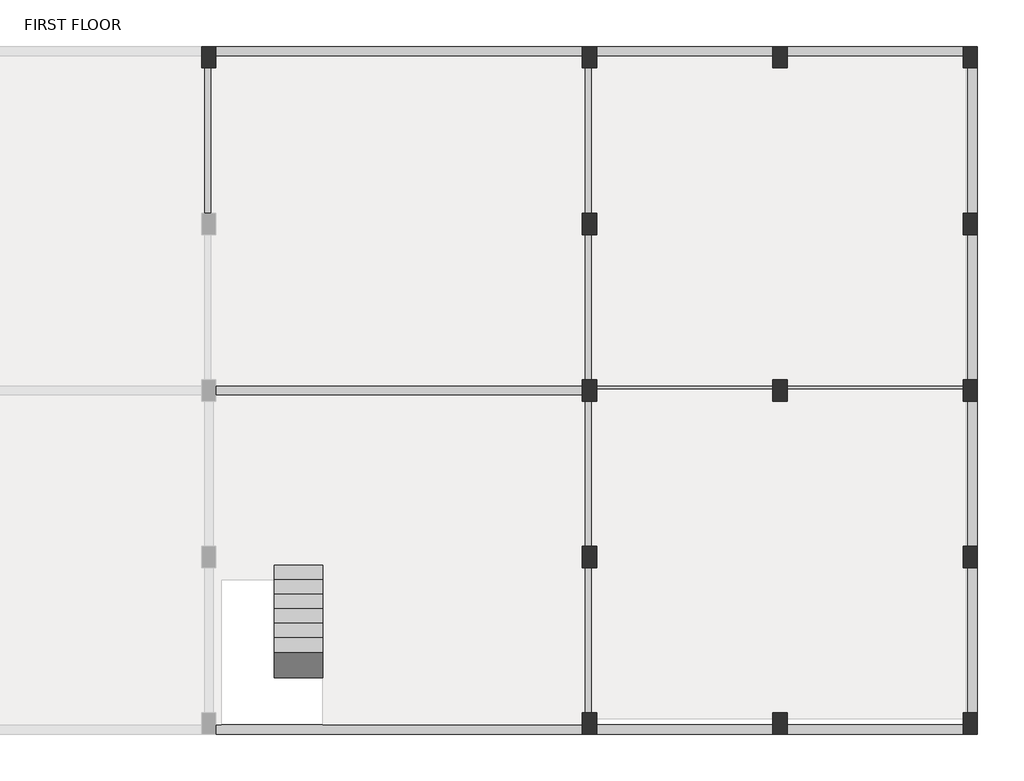
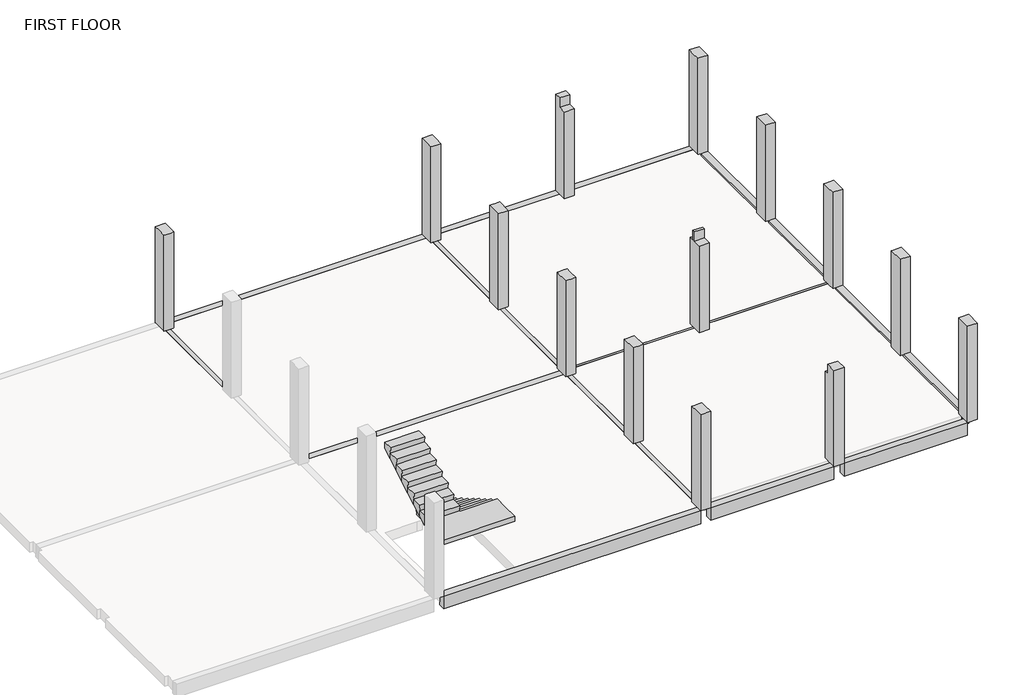
# One storey, part 2 of 2: 18 beams, 14 columns, 1 stair flight.
"""IFC4 building model written with IfcOpenShell, lengths in millimetres."""

from ifc_helpers import new_model, si_unit, frame, origin, place, context, project, spatial, polyline, outline, extrude, faceted_brep, element, save

model = new_model("IFC4")

# Units and contexts
model_context = context("Model", 3, world=origin())
ifc_project = project(units=[si_unit("LENGTHUNIT", "METRE", prefix="MILLI")], contexts=[model_context])

# Site, building, storey
site = spatial("IfcSite", under=ifc_project)
building = spatial("IfcBuilding", under=site)
storey = spatial("IfcBuildingStorey", under=building, Name="FIRST FLOOR", Elevation=3048.0)

# Beams
placement = place(None, origin())
element("IfcBeam", 1, ObjectType="M_Concrete-Rectangular Beam : 200MMX400MM", at=placement, inside=storey, context=model_context, shape_type="Brep", body=[
    faceted_brep([(4019.3125983, 15797.7008557, 3048.0), (4019.3125983, 15997.7008557, 3048.0), (-3680.6874017, 15997.7008557, 3048.0), (-3680.6874017, 15797.7008557, 3048.0), (4019.3125983, 15797.7008557, 2648.0), (4019.3125983, 15797.7008557, 2748.0), (-3680.6874017, 15797.7008557, 2748.0), (-3680.6874017, 15797.7008557, 2648.0), (4019.3125983, 15997.7008557, 2648.0), (-3680.6874017, 15997.7008557, 2648.0)], [[[0, 1, 2, 3]], [[4, 5, 0, 3, 6, 7]], [[8, 4, 7, 9]], [[1, 8, 9, 2]], [[1, 0, 5, 4, 8]], [[2, 9, 7, 6, 3]]]),
])
element("IfcBeam", 2, ObjectType="M_Concrete-Rectangular Beam : 200MMX400MM", at=placement, inside=storey, context=model_context, shape_type="Brep", body=[
    faceted_brep([(8019.3125983, 15797.7008557, 3048.0), (8019.3125983, 15997.7008557, 3048.0), (4319.3125983, 15997.7008557, 3048.0), (4319.3125983, 15797.7008557, 3048.0), (8019.3125983, 15797.7008557, 2648.0), (4319.3125983, 15797.7008557, 2748.0), (4319.3125983, 15797.7008557, 2648.0), (8019.3125983, 15997.7008557, 2648.0), (4319.3125983, 15997.7008557, 2648.0)], [[[0, 1, 2, 3]], [[4, 0, 3, 5, 6]], [[7, 4, 6, 8]], [[1, 7, 8, 2]], [[2, 8, 6, 5, 3]], [[1, 0, 4, 7]]]),
])
element("IfcBeam", 3, ObjectType="M_Concrete-Rectangular Beam : 200MMX400MM", at=placement, inside=storey, context=model_context, shape_type="Brep", body=[
    faceted_brep([(12019.3125983, 15797.7008557, 3048.0), (12019.3125983, 15997.7008557, 3048.0), (8319.3125983, 15997.7008557, 3048.0), (8319.3125983, 15797.7008557, 3048.0), (12019.3125983, 15797.7008557, 2648.0), (12019.3125983, 15797.7008557, 2748.0), (8319.3125983, 15797.7008557, 2648.0), (12019.3125983, 15997.7008557, 2648.0), (8319.3125983, 15997.7008557, 2648.0)], [[[0, 1, 2, 3]], [[4, 5, 0, 3, 6]], [[7, 4, 6, 8]], [[1, 7, 8, 2]], [[2, 8, 6, 3]], [[1, 0, 5, 4, 7]]]),
])
element("IfcBeam", 4, ObjectType="M_Concrete-Rectangular Beam : 200MMX400MM", at=placement, inside=storey, context=model_context, shape_type="SweptSolid", body=[
    extrude(outline(polyline([(12319.3125983, 12497.7008557), (12119.3125983, 12497.7008557), (12119.3125983, 15547.7008557), (12319.3125983, 15547.7008557), (12319.3125983, 12497.7008557)])), frame((0.0, 0.0, 2648.0), z_axis=(0.0, 0.0, 1.0), x_axis=(1.0, 0.0, 0.0)), (0.0, 0.0, 1.0), 400.0),
])
element("IfcBeam", 5, ObjectType="M_Concrete-Rectangular Beam : 200MMX400MM", at=placement, inside=storey, context=model_context, shape_type="SweptSolid", body=[
    extrude(outline(polyline([(12319.3125983, 1997.7008557), (12119.3125983, 1997.7008557), (12119.3125983, 5047.7008557), (12319.3125983, 5047.7008557), (12319.3125983, 1997.7008557)])), frame((0.0, 0.0, 2648.0), z_axis=(0.0, 0.0, 1.0), x_axis=(1.0, 0.0, 0.0)), (0.0, 0.0, 1.0), 400.0),
])
element("IfcBeam", 6, ObjectType="M_Concrete-Rectangular Beam : 200MMX400MM", at=placement, inside=storey, context=model_context, shape_type="SweptSolid", body=[
    extrude(outline(polyline([(8319.3125983, 1547.7008557), (8319.3125983, 1747.7008557), (12019.3125983, 1747.7008557), (12019.3125983, 1547.7008557), (8319.3125983, 1547.7008557)])), frame((0.0, 0.0, 2648.0), z_axis=(0.0, 0.0, 1.0), x_axis=(1.0, 0.0, 0.0)), (0.0, 0.0, 1.0), 400.0),
])
element("IfcBeam", 7, ObjectType="M_Concrete-Rectangular Beam : 200MMX400MM", at=placement, inside=storey, context=model_context, shape_type="SweptSolid", body=[
    extrude(outline(polyline([(8019.3125983, 1747.7008557), (8019.3125983, 1547.7008557), (4319.3125983, 1547.7008557), (4319.3125983, 1747.7008557), (8019.3125983, 1747.7008557)])), frame((0.0, 0.0, 2648.0), z_axis=(0.0, 0.0, 1.0), x_axis=(1.0, 0.0, 0.0)), (0.0, 0.0, 1.0), 400.0),
])
element("IfcBeam", 8, ObjectType="M_Concrete-Rectangular Beam : 200MMX400MM", at=placement, inside=storey, context=model_context, shape_type="Brep", body=[
    faceted_brep([(-3680.6874017, 1747.7008557, 3048.0), (-3680.6874017, 1547.7008557, 3048.0), (4019.3125983, 1547.7008557, 3048.0), (4019.3125983, 1747.7008557, 3048.0), (-1437.0874017, 1747.7008557, 3048.0), (-3570.6874017, 1747.7008557, 3048.0), (-3680.6874017, 1747.7008557, 2648.0), (-3680.6874017, 1747.7008557, 2748.0), (4019.3125983, 1747.7008557, 2748.0), (4019.3125983, 1747.7008557, 2648.0), (-3680.6874017, 1547.7008557, 2648.0), (4019.3125983, 1547.7008557, 2648.0)], [[[0, 1, 2, 3, 4, 5]], [[6, 7, 0, 5, 4, 3, 8, 9]], [[10, 6, 9, 11]], [[1, 10, 11, 2]], [[1, 0, 7, 6, 10]], [[2, 11, 9, 8, 3]]]),
])
element("IfcBeam", 9, ObjectType="M_Concrete-Rectangular Beam : 200MMX400MM", at=placement, inside=storey, context=model_context, shape_type="Brep", body=[
    faceted_brep([(4019.3125983, 8872.7008557, 3048.0), (-3680.6874017, 8872.7008557, 3048.0), (-3680.6874017, 8672.7008557, 3048.0), (4019.3125983, 8672.7008557, 3048.0), (-3680.6874017, 8672.7008557, 2748.0), (-3680.6874017, 8672.7008557, 2648.0), (4019.3125983, 8672.7008557, 2648.0), (4019.3125983, 8672.7008557, 2748.0), (-3680.6874017, 8872.7008557, 2648.0), (4019.3125983, 8872.7008557, 2648.0), (4019.3125983, 8872.7008557, 2748.0), (-3680.6874017, 8872.7008557, 2748.0)], [[[0, 1, 2, 3]], [[3, 2, 4, 5, 6, 7]], [[6, 5, 8, 9]], [[1, 0, 10, 9, 8, 11]], [[8, 5, 4, 2, 1, 11]], [[0, 3, 7, 6, 9, 10]]]),
])
element("IfcBeam", 10, ObjectType="M_Concrete-Rectangular Beam : 200MMX400MM", at=placement, inside=storey, context=model_context, shape_type="Brep", body=[
    faceted_brep([(8019.3125983, 8872.7008557, 3048.0), (4319.3125983, 8872.7008557, 3048.0), (4319.3125983, 8797.7008557, 3048.0), (8019.3125983, 8797.7008557, 3048.0), (4319.3125983, 8672.7008557, 2648.0), (8019.3125983, 8672.7008557, 2648.0), (8019.3125983, 8672.7008557, 2748.0), (4319.3125983, 8672.7008557, 2748.0), (4319.3125983, 8872.7008557, 2648.0), (8019.3125983, 8872.7008557, 2648.0), (8019.3125983, 8872.7008557, 2748.0), (4319.3125983, 8872.7008557, 2748.0), (4319.3125983, 8797.7008557, 2748.0), (8019.3125983, 8797.7008557, 2748.0)], [[[0, 1, 2, 3]], [[4, 5, 6, 7]], [[5, 4, 8, 9]], [[1, 0, 10, 9, 8, 11]], [[8, 4, 7, 12, 2, 1, 11]], [[5, 9, 10, 0, 3, 13, 6]], [[13, 12, 7, 6]], [[12, 13, 3, 2]]]),
])
element("IfcBeam", 11, ObjectType="M_Concrete-Rectangular Beam : 200MMX400MM", at=placement, inside=storey, context=model_context, shape_type="Brep", body=[
    faceted_brep([(12019.3125983, 8872.7008557, 3048.0), (8319.3125983, 8872.7008557, 3048.0), (8319.3125983, 8797.7008557, 3048.0), (12019.3125983, 8797.7008557, 3048.0), (8319.3125983, 8672.7008557, 2648.0), (12019.3125983, 8672.7008557, 2648.0), (12019.3125983, 8672.7008557, 2748.0), (8319.3125983, 8672.7008557, 2748.0), (8319.3125983, 8872.7008557, 2648.0), (12019.3125983, 8872.7008557, 2648.0), (12019.3125983, 8872.7008557, 2748.0), (8319.3125983, 8872.7008557, 2748.0), (12019.3125983, 8797.7008557, 2748.0), (8319.3125983, 8797.7008557, 2748.0)], [[[0, 1, 2, 3]], [[4, 5, 6, 7]], [[5, 4, 8, 9]], [[1, 0, 10, 9, 8, 11]], [[5, 9, 10, 0, 3, 12, 6]], [[8, 4, 7, 13, 2, 1, 11]], [[12, 13, 7, 6]], [[13, 12, 3, 2]]]),
])
element("IfcBeam", 12, ObjectType="M_Concrete-Rectangular Beam : 200MMX400MM", at=placement, inside=storey, context=model_context, shape_type="SweptSolid", body=[
    extrude(outline(polyline([(12319.3125983, 5497.7008557), (12119.3125983, 5497.7008557), (12119.3125983, 8547.7008557), (12319.3125983, 8547.7008557), (12319.3125983, 5497.7008557)])), frame((0.0, 0.0, 2648.0), z_axis=(0.0, 0.0, 1.0), x_axis=(1.0, 0.0, 0.0)), (0.0, 0.0, 1.0), 400.0),
])
element("IfcBeam", 13, ObjectType="M_Concrete-Rectangular Beam : 200MMX400MM", at=placement, inside=storey, context=model_context, shape_type="SweptSolid", body=[
    extrude(outline(polyline([(12119.3125983, 12047.7008557), (12319.3125983, 12047.7008557), (12319.3125983, 8997.7008557), (12119.3125983, 8997.7008557), (12119.3125983, 12047.7008557)])), frame((0.0, 0.0, 2648.0), z_axis=(0.0, 0.0, 1.0), x_axis=(1.0, 0.0, 0.0)), (0.0, 0.0, 1.0), 400.0),
])
element("IfcBeam", 14, ObjectType="M_Concrete-Rectangular Beam : 200MMX400MM", at=placement, inside=storey, context=model_context, shape_type="Brep", body=[
    faceted_brep([(4069.3125983, 5047.7008557, 3048.0), (4069.3125983, 1997.7008557, 3048.0), (4219.3125983, 1997.7008557, 3048.0), (4219.3125983, 5047.7008557, 3048.0), (4269.3125983, 1997.7008557, 2648.0), (4269.3125983, 5047.7008557, 2648.0), (4269.3125983, 5047.7008557, 2748.0), (4269.3125983, 1997.7008557, 2748.0), (4069.3125983, 1997.7008557, 2648.0), (4069.3125983, 5047.7008557, 2648.0), (4069.3125983, 5047.7008557, 2748.0), (4069.3125983, 1997.7008557, 2748.0), (4219.3125983, 1997.7008557, 2748.0), (4219.3125983, 5047.7008557, 2748.0)], [[[0, 1, 2, 3]], [[4, 5, 6, 7]], [[5, 4, 8, 9]], [[1, 0, 10, 9, 8, 11]], [[8, 4, 7, 12, 2, 1, 11]], [[5, 9, 10, 0, 3, 13, 6]], [[13, 12, 7, 6]], [[12, 13, 3, 2]]]),
])
element("IfcBeam", 15, ObjectType="M_Concrete-Rectangular Beam : 200MMX400MM", at=placement, inside=storey, context=model_context, shape_type="Brep", body=[
    faceted_brep([(4069.3125983, 8547.7008557, 3048.0), (4069.3125983, 5497.7008557, 3048.0), (4219.3125983, 5497.7008557, 3048.0), (4219.3125983, 8547.7008557, 3048.0), (4269.3125983, 5497.7008557, 2648.0), (4269.3125983, 8547.7008557, 2648.0), (4269.3125983, 8547.7008557, 2748.0), (4269.3125983, 5497.7008557, 2748.0), (4069.3125983, 5497.7008557, 2648.0), (4069.3125983, 8547.7008557, 2648.0), (4069.3125983, 8547.7008557, 2748.0), (4069.3125983, 5497.7008557, 2748.0), (4219.3125983, 8547.7008557, 2748.0), (4219.3125983, 5497.7008557, 2748.0)], [[[0, 1, 2, 3]], [[4, 5, 6, 7]], [[5, 4, 8, 9]], [[1, 0, 10, 9, 8, 11]], [[5, 9, 10, 0, 3, 12, 6]], [[8, 4, 7, 13, 2, 1, 11]], [[12, 13, 7, 6]], [[13, 12, 3, 2]]]),
])
element("IfcBeam", 16, ObjectType="M_Concrete-Rectangular Beam : 200MMX400MM", at=placement, inside=storey, context=model_context, shape_type="Brep", body=[
    faceted_brep([(4069.3125983, 12047.7008557, 3048.0), (4069.3125983, 8997.7008557, 3048.0), (4219.3125983, 8997.7008557, 3048.0), (4219.3125983, 12047.7008557, 3048.0), (4269.3125983, 8997.7008557, 2648.0), (4269.3125983, 12047.7008557, 2648.0), (4269.3125983, 12047.7008557, 2748.0), (4269.3125983, 8997.7008557, 2748.0), (4069.3125983, 8997.7008557, 2648.0), (4069.3125983, 12047.7008557, 2648.0), (4069.3125983, 12047.7008557, 2748.0), (4069.3125983, 8997.7008557, 2748.0), (4219.3125983, 8997.7008557, 2748.0), (4219.3125983, 12047.7008557, 2748.0)], [[[0, 1, 2, 3]], [[4, 5, 6, 7]], [[5, 4, 8, 9]], [[1, 0, 10, 9, 8, 11]], [[8, 4, 7, 12, 2, 1, 11]], [[5, 9, 10, 0, 3, 13, 6]], [[13, 12, 7, 6]], [[12, 13, 3, 2]]]),
])
element("IfcBeam", 17, ObjectType="M_Concrete-Rectangular Beam : 200MMX400MM", at=placement, inside=storey, context=model_context, shape_type="Brep", body=[
    faceted_brep([(4069.3125983, 15547.7008557, 3048.0), (4069.3125983, 12497.7008557, 3048.0), (4219.3125983, 12497.7008557, 3048.0), (4219.3125983, 15547.7008557, 3048.0), (4269.3125983, 12497.7008557, 2648.0), (4269.3125983, 15547.7008557, 2648.0), (4269.3125983, 15547.7008557, 2748.0), (4269.3125983, 12497.7008557, 2748.0), (4069.3125983, 12497.7008557, 2648.0), (4069.3125983, 15547.7008557, 2648.0), (4069.3125983, 15547.7008557, 2748.0), (4069.3125983, 12497.7008557, 2748.0), (4219.3125983, 15547.7008557, 2748.0), (4219.3125983, 12497.7008557, 2748.0)], [[[0, 1, 2, 3]], [[4, 5, 6, 7]], [[5, 4, 8, 9]], [[1, 0, 10, 9, 8, 11]], [[5, 9, 10, 0, 3, 12, 6]], [[8, 4, 7, 13, 2, 1, 11]], [[12, 13, 7, 6]], [[13, 12, 3, 2]]]),
])
element("IfcBeam", 18, ObjectType="M_Concrete-Rectangular Beam : 200MMX400MM", at=placement, inside=storey, context=model_context, shape_type="Brep", body=[
    faceted_brep([(-3930.6874017, 15547.7008557, 3048.0), (-3930.6874017, 12497.7008557, 3048.0), (-3780.6874017, 12497.7008557, 3048.0), (-3780.6874017, 15547.7008557, 3048.0), (-3730.6874017, 12497.7008557, 2648.0), (-3730.6874017, 15547.7008557, 2648.0), (-3730.6874017, 15547.7008557, 2748.0), (-3730.6874017, 12497.7008557, 2748.0), (-3930.6874017, 12497.7008557, 2648.0), (-3930.6874017, 15547.7008557, 2648.0), (-3930.6874017, 15547.7008557, 2748.0), (-3930.6874017, 12497.7008557, 2748.0), (-3780.6874017, 15547.7008557, 2748.0), (-3780.6874017, 12497.7008557, 2748.0)], [[[0, 1, 2, 3]], [[4, 5, 6, 7]], [[5, 4, 8, 9]], [[1, 0, 10, 9, 8, 11]], [[5, 9, 10, 0, 3, 12, 6]], [[8, 4, 7, 13, 2, 1, 11]], [[12, 13, 7, 6]], [[13, 12, 3, 2]]]),
])

# Columns
element("IfcColumn", 19, ObjectType="M_Concrete-Rectangular-Column : 300 x 450mm", at=placement, inside=storey, context=model_context, shape_type="Brep", body=[
    faceted_brep([(-3680.6874017, 15997.7008557, 3048.0), (-3680.6874017, 15547.7008557, 3048.0), (-3980.6874017, 15547.7008557, 3048.0), (-3980.6874017, 15997.7008557, 3048.0), (-3680.6874017, 15997.7008557, 6096.0), (-3680.6874017, 15797.7008557, 6096.0), (-3680.6874017, 15547.7008557, 6096.0), (-3680.6874017, 15547.7008557, 5796.0), (-3780.6874017, 15547.7008557, 6096.0), (-3930.6874017, 15547.7008557, 6096.0), (-3980.6874017, 15547.7008557, 6096.0), (-3980.6874017, 15547.7008557, 5796.0), (-3980.6874017, 15797.7008557, 6096.0), (-3980.6874017, 15997.7008557, 6096.0)], [[[0, 1, 2, 3]], [[1, 0, 4, 5, 6, 7]], [[2, 1, 7, 6, 8, 9, 10, 11]], [[3, 2, 11, 10, 12, 13]], [[0, 3, 13, 4]], [[4, 13, 12, 10, 9, 8, 6, 5]]]),
])
element("IfcColumn", 20, ObjectType="M_Concrete-Rectangular-Column : 300 x 450mm", at=placement, inside=storey, context=model_context, shape_type="Brep", body=[
    faceted_brep([(4319.3125983, 15997.7008557, 3048.0), (4319.3125983, 15547.7008557, 3048.0), (4019.3125983, 15547.7008557, 3048.0), (4019.3125983, 15997.7008557, 3048.0), (4319.3125983, 15997.7008557, 6096.0), (4319.3125983, 15797.7008557, 6096.0), (4319.3125983, 15547.7008557, 6096.0), (4319.3125983, 15547.7008557, 5796.0), (4219.3125983, 15547.7008557, 6096.0), (4069.3125983, 15547.7008557, 6096.0), (4019.3125983, 15547.7008557, 6096.0), (4019.3125983, 15547.7008557, 5796.0), (4019.3125983, 15797.7008557, 6096.0), (4019.3125983, 15997.7008557, 6096.0)], [[[0, 1, 2, 3]], [[1, 0, 4, 5, 6, 7]], [[2, 1, 7, 6, 8, 9, 10, 11]], [[3, 2, 11, 10, 12, 13]], [[0, 3, 13, 4]], [[4, 13, 12, 10, 9, 8, 6, 5]]]),
])
element("IfcColumn", 21, ObjectType="M_Concrete-Rectangular-Column : 300 x 450mm", at=placement, inside=storey, context=model_context, shape_type="Brep", body=[
    faceted_brep([(4319.3125983, 8997.7008557, 3048.0), (4319.3125983, 8547.7008557, 3048.0), (4019.3125983, 8547.7008557, 3048.0), (4019.3125983, 8997.7008557, 3048.0), (4319.3125983, 8997.7008557, 5796.0), (4319.3125983, 8997.7008557, 6096.0), (4319.3125983, 8872.7008557, 6096.0), (4319.3125983, 8797.7008557, 6096.0), (4319.3125983, 8547.7008557, 6096.0), (4319.3125983, 8547.7008557, 5796.0), (4219.3125983, 8547.7008557, 6096.0), (4069.3125983, 8547.7008557, 6096.0), (4019.3125983, 8547.7008557, 6096.0), (4019.3125983, 8547.7008557, 5796.0), (4019.3125983, 8672.7008557, 6096.0), (4019.3125983, 8872.7008557, 6096.0), (4019.3125983, 8997.7008557, 6096.0), (4019.3125983, 8997.7008557, 5796.0), (4069.3125983, 8997.7008557, 6096.0), (4219.3125983, 8997.7008557, 6096.0)], [[[0, 1, 2, 3]], [[1, 0, 4, 5, 6, 7, 8, 9]], [[2, 1, 9, 8, 10, 11, 12, 13]], [[3, 2, 13, 12, 14, 15, 16, 17]], [[0, 3, 17, 16, 18, 19, 5, 4]], [[18, 16, 15, 14, 12, 11, 10, 8, 7, 6, 5, 19]]]),
])
element("IfcColumn", 22, ObjectType="M_Concrete-Rectangular-Column : 300 x 450mm", at=placement, inside=storey, context=model_context, shape_type="Brep", body=[
    faceted_brep([(4319.3125983, 1997.7008557, 3048.0), (4319.3125983, 1547.7008557, 3048.0), (4019.3125983, 1547.7008557, 3048.0), (4019.3125983, 1997.7008557, 3048.0), (4319.3125983, 1997.7008557, 5796.0), (4319.3125983, 1997.7008557, 6096.0), (4319.3125983, 1872.7008557, 6096.0), (4319.3125983, 1547.7008557, 6096.0), (4019.3125983, 1547.7008557, 6096.0), (4019.3125983, 1747.7008557, 6096.0), (4019.3125983, 1997.7008557, 6096.0), (4019.3125983, 1997.7008557, 5796.0), (4069.3125983, 1997.7008557, 6096.0), (4219.3125983, 1997.7008557, 6096.0)], [[[0, 1, 2, 3]], [[1, 0, 4, 5, 6, 7]], [[2, 1, 7, 8]], [[3, 2, 8, 9, 10, 11]], [[0, 3, 11, 10, 12, 13, 5, 4]], [[8, 7, 6, 5, 13, 12, 10, 9]]]),
])
element("IfcColumn", 23, ObjectType="M_Concrete-Rectangular-Column : 300 x 450mm", at=placement, inside=storey, context=model_context, shape_type="SweptSolid", body=[
    extrude(outline(polyline([(15997.7008557, 3048.0), (15547.7008557, 3048.0), (15547.7008557, 5796.0), (15797.7008557, 5796.0), (15797.7008557, 6096.0), (15997.7008557, 6096.0), (15997.7008557, 3048.0)])), frame((8019.3125983, 0.0, 0.0), z_axis=(1.0, 0.0, 0.0), x_axis=(0.0, 1.0, 0.0)), (0.0, 0.0, 1.0), 300.0),
])
element("IfcColumn", 24, ObjectType="M_Concrete-Rectangular-Column : 300 x 450mm", at=placement, inside=storey, context=model_context, shape_type="SweptSolid", body=[
    extrude(outline(polyline([(1997.7008557, 3048.0), (1547.7008557, 3048.0), (1547.7008557, 6096.0), (1872.7008557, 6096.0), (1872.7008557, 5796.0), (1997.7008557, 5796.0), (1997.7008557, 3048.0)])), frame((8019.3125983, 0.0, 0.0), z_axis=(1.0, 0.0, 0.0), x_axis=(0.0, 1.0, 0.0)), (0.0, 0.0, 1.0), 300.0),
])
element("IfcColumn", 25, ObjectType="M_Concrete-Rectangular-Column : 300 x 450mm", at=placement, inside=storey, context=model_context, shape_type="Brep", body=[
    faceted_brep([(12319.3125983, 12497.7008557, 3048.0), (12319.3125983, 12047.7008557, 3048.0), (12019.3125983, 12047.7008557, 3048.0), (12019.3125983, 12497.7008557, 3048.0), (12319.3125983, 12497.7008557, 6096.0), (12319.3125983, 12047.7008557, 6096.0), (12069.3125983, 12047.7008557, 6096.0), (12019.3125983, 12047.7008557, 6096.0), (12019.3125983, 12047.7008557, 5796.0), (12019.3125983, 12497.7008557, 6096.0), (12019.3125983, 12497.7008557, 5796.0), (12069.3125983, 12497.7008557, 6096.0)], [[[0, 1, 2, 3]], [[1, 0, 4, 5]], [[2, 1, 5, 6, 7, 8]], [[3, 2, 8, 7, 9, 10]], [[0, 3, 10, 9, 11, 4]], [[5, 4, 11, 9, 7, 6]]]),
])
element("IfcColumn", 26, ObjectType="M_Concrete-Rectangular-Column : 300 x 450mm", at=placement, inside=storey, context=model_context, shape_type="Brep", body=[
    faceted_brep([(12319.3125983, 5497.7008557, 3048.0), (12319.3125983, 5047.7008557, 3048.0), (12019.3125983, 5047.7008557, 3048.0), (12019.3125983, 5497.7008557, 3048.0), (12319.3125983, 5497.7008557, 6096.0), (12319.3125983, 5047.7008557, 6096.0), (12069.3125983, 5047.7008557, 6096.0), (12019.3125983, 5047.7008557, 6096.0), (12019.3125983, 5047.7008557, 5796.0), (12019.3125983, 5497.7008557, 6096.0), (12019.3125983, 5497.7008557, 5796.0), (12069.3125983, 5497.7008557, 6096.0)], [[[0, 1, 2, 3]], [[1, 0, 4, 5]], [[2, 1, 5, 6, 7, 8]], [[3, 2, 8, 7, 9, 10]], [[0, 3, 10, 9, 11, 4]], [[5, 4, 11, 9, 7, 6]]]),
])
element("IfcColumn", 27, ObjectType="M_Concrete-Rectangular-Column : 300 x 450mm", at=placement, inside=storey, context=model_context, shape_type="Brep", body=[
    faceted_brep([(12319.3125983, 15997.7008557, 3048.0), (12319.3125983, 15547.7008557, 3048.0), (12019.3125983, 15547.7008557, 3048.0), (12019.3125983, 15997.7008557, 3048.0), (12319.3125983, 15997.7008557, 6096.0), (12319.3125983, 15547.7008557, 6096.0), (12069.3125983, 15547.7008557, 6096.0), (12019.3125983, 15547.7008557, 6096.0), (12019.3125983, 15547.7008557, 5796.0), (12019.3125983, 15797.7008557, 6096.0), (12019.3125983, 15997.7008557, 6096.0)], [[[0, 1, 2, 3]], [[1, 0, 4, 5]], [[2, 1, 5, 6, 7, 8]], [[3, 2, 8, 7, 9, 10]], [[0, 3, 10, 4]], [[5, 4, 10, 9, 7, 6]]]),
])
element("IfcColumn", 28, ObjectType="M_Concrete-Rectangular-Column : 300 x 450mm", at=placement, inside=storey, context=model_context, shape_type="Brep", body=[
    faceted_brep([(12319.3125983, 1997.7008557, 3048.0), (12319.3125983, 1547.7008557, 3048.0), (12019.3125983, 1547.7008557, 3048.0), (12019.3125983, 1997.7008557, 3048.0), (12319.3125983, 1997.7008557, 6096.0), (12319.3125983, 1547.7008557, 6096.0), (12019.3125983, 1547.7008557, 6096.0), (12019.3125983, 1872.7008557, 6096.0), (12019.3125983, 1997.7008557, 6096.0), (12019.3125983, 1997.7008557, 5796.0), (12069.3125983, 1997.7008557, 6096.0)], [[[0, 1, 2, 3]], [[1, 0, 4, 5]], [[2, 1, 5, 6]], [[3, 2, 6, 7, 8, 9]], [[0, 3, 9, 8, 10, 4]], [[5, 4, 10, 8, 7, 6]]]),
])
element("IfcColumn", 29, ObjectType="M_Concrete-Rectangular-Column : 300 x 450mm", at=placement, inside=storey, context=model_context, shape_type="Brep", body=[
    faceted_brep([(12319.3125983, 8997.7008557, 3048.0), (12319.3125983, 8547.7008557, 3048.0), (12019.3125983, 8547.7008557, 3048.0), (12019.3125983, 8997.7008557, 3048.0), (12319.3125983, 8997.7008557, 6096.0), (12319.3125983, 8547.7008557, 6096.0), (12069.3125983, 8547.7008557, 6096.0), (12019.3125983, 8547.7008557, 6096.0), (12019.3125983, 8547.7008557, 5796.0), (12019.3125983, 8797.7008557, 6096.0), (12019.3125983, 8872.7008557, 6096.0), (12019.3125983, 8997.7008557, 6096.0), (12019.3125983, 8997.7008557, 5796.0), (12069.3125983, 8997.7008557, 6096.0)], [[[0, 1, 2, 3]], [[1, 0, 4, 5]], [[2, 1, 5, 6, 7, 8]], [[3, 2, 8, 7, 9, 10, 11, 12]], [[0, 3, 12, 11, 13, 4]], [[5, 4, 13, 11, 10, 9, 7, 6]]]),
])
element("IfcColumn", 30, ObjectType="M_Concrete-Rectangular-Column : 300 x 450mm", at=placement, inside=storey, context=model_context, shape_type="Brep", body=[
    faceted_brep([(8319.3125983, 8997.7008557, 3048.0), (8319.3125983, 8547.7008557, 3048.0), (8019.3125983, 8547.7008557, 3048.0), (8019.3125983, 8997.7008557, 3048.0), (8319.3125983, 8997.7008557, 5796.0), (8319.3125983, 8872.7008557, 5796.0), (8319.3125983, 8872.7008557, 6096.0), (8319.3125983, 8797.7008557, 6096.0), (8319.3125983, 8797.7008557, 5796.0), (8319.3125983, 8547.7008557, 5796.0), (8019.3125983, 8547.7008557, 5796.0), (8019.3125983, 8672.7008557, 5796.0), (8019.3125983, 8797.7008557, 5796.0), (8019.3125983, 8797.7008557, 6096.0), (8019.3125983, 8872.7008557, 6096.0), (8019.3125983, 8872.7008557, 5796.0), (8019.3125983, 8997.7008557, 5796.0)], [[[0, 1, 2, 3]], [[1, 0, 4, 5, 6, 7, 8, 9]], [[2, 1, 9, 10]], [[3, 2, 10, 11, 12, 13, 14, 15, 16]], [[0, 3, 16, 4]], [[14, 13, 7, 6]], [[8, 12, 11, 10, 9]], [[5, 15, 14, 6]], [[12, 8, 7, 13]], [[15, 5, 4, 16]]]),
])
element("IfcColumn", 31, ObjectType="M_Concrete-Rectangular-Column : 300 x 450mm", at=placement, inside=storey, context=model_context, shape_type="Brep", body=[
    faceted_brep([(4319.3125983, 12497.7008557, 3048.0), (4319.3125983, 12047.7008557, 3048.0), (4019.3125983, 12047.7008557, 3048.0), (4019.3125983, 12497.7008557, 3048.0), (4319.3125983, 12497.7008557, 5796.0), (4319.3125983, 12497.7008557, 6096.0), (4319.3125983, 12047.7008557, 6096.0), (4319.3125983, 12047.7008557, 5796.0), (4219.3125983, 12047.7008557, 6096.0), (4069.3125983, 12047.7008557, 6096.0), (4019.3125983, 12047.7008557, 6096.0), (4019.3125983, 12047.7008557, 5796.0), (4019.3125983, 12497.7008557, 6096.0), (4019.3125983, 12497.7008557, 5796.0), (4069.3125983, 12497.7008557, 6096.0), (4219.3125983, 12497.7008557, 6096.0)], [[[0, 1, 2, 3]], [[1, 0, 4, 5, 6, 7]], [[2, 1, 7, 6, 8, 9, 10, 11]], [[3, 2, 11, 10, 12, 13]], [[0, 3, 13, 12, 14, 15, 5, 4]], [[6, 5, 15, 14, 12, 10, 9, 8]]]),
])
element("IfcColumn", 32, ObjectType="M_Concrete-Rectangular-Column : 300 x 450mm", at=placement, inside=storey, context=model_context, shape_type="Brep", body=[
    faceted_brep([(4319.3125983, 5497.7008557, 3048.0), (4319.3125983, 5047.7008557, 3048.0), (4019.3125983, 5047.7008557, 3048.0), (4019.3125983, 5497.7008557, 3048.0), (4319.3125983, 5497.7008557, 5796.0), (4319.3125983, 5497.7008557, 6096.0), (4319.3125983, 5047.7008557, 6096.0), (4319.3125983, 5047.7008557, 5796.0), (4219.3125983, 5047.7008557, 6096.0), (4069.3125983, 5047.7008557, 6096.0), (4019.3125983, 5047.7008557, 6096.0), (4019.3125983, 5047.7008557, 5796.0), (4019.3125983, 5497.7008557, 6096.0), (4019.3125983, 5497.7008557, 5796.0), (4069.3125983, 5497.7008557, 6096.0), (4219.3125983, 5497.7008557, 6096.0)], [[[0, 1, 2, 3]], [[1, 0, 4, 5, 6, 7]], [[2, 1, 7, 6, 8, 9, 10, 11]], [[3, 2, 11, 10, 12, 13]], [[0, 3, 13, 12, 14, 15, 5, 4]], [[6, 5, 15, 14, 12, 10, 9, 8]]]),
])

# Stair flight
element("IfcStairFlight", 33, ObjectType="25 mm Nosing", at=placement, inside=storey, context=model_context, shape_type="Brep", body=[
    faceted_brep([(-1437.0874017, 5100.5008557, 3227.2941176), (-2453.0874017, 5100.5008557, 3227.2941176), (-2453.0874017, 4770.7008557, 3227.2941176), (-1437.0874017, 4770.7008557, 3227.2941176), (-1437.0874017, 4770.7008557, 3053.2669154), (-1437.0874017, 4779.6546118, 3048.0), (-1437.0874017, 5075.5008557, 3048.0), (-2453.0874017, 5075.5008557, 3048.0), (-2453.0874017, 4779.6546118, 3048.0), (-2453.0874017, 4770.7008557, 3053.2669154), (-1437.0874017, 4795.7008557, 3406.5882353), (-2453.0874017, 4795.7008557, 3406.5882353), (-2453.0874017, 4465.9008557, 3406.5882353), (-1437.0874017, 4465.9008557, 3406.5882353), (-1437.0874017, 4465.9008557, 3232.561033), (-2453.0874017, 4465.9008557, 3232.561033), (-1437.0874017, 4490.9008557, 3585.8823529), (-2453.0874017, 4490.9008557, 3585.8823529), (-2453.0874017, 4161.1008557, 3585.8823529), (-1437.0874017, 4161.1008557, 3585.8823529), (-1437.0874017, 4161.1008557, 3411.8551507), (-2453.0874017, 4161.1008557, 3411.8551507), (-1437.0874017, 4186.1008557, 3765.1764706), (-2453.0874017, 4186.1008557, 3765.1764706), (-2453.0874017, 3856.3008557, 3765.1764706), (-1437.0874017, 3856.3008557, 3765.1764706), (-1437.0874017, 3856.3008557, 3591.1492683), (-2453.0874017, 3856.3008557, 3591.1492683), (-1437.0874017, 3881.3008557, 3944.4705882), (-2453.0874017, 3881.3008557, 3944.4705882), (-2453.0874017, 3551.5008557, 3944.4705882), (-1437.0874017, 3551.5008557, 3944.4705882), (-1437.0874017, 3551.5008557, 3770.443386), (-2453.0874017, 3551.5008557, 3770.443386), (-1437.0874017, 3576.5008557, 4123.7647059), (-2453.0874017, 3576.5008557, 4123.7647059), (-2453.0874017, 3246.7008557, 4123.7647059), (-1437.0874017, 3246.7008557, 4123.7647059), (-1437.0874017, 3246.7008557, 3949.7375036), (-2453.0874017, 3246.7008557, 3949.7375036), (-1437.0874017, 3271.7008557, 4303.0588235), (-2453.0874017, 3271.7008557, 4303.0588235), (-2453.0874017, 2941.9008557, 4303.0588235), (-1437.0874017, 2941.9008557, 4303.0588235), (-1437.0874017, 2941.9008557, 4129.0316213), (-2453.0874017, 2941.9008557, 4129.0316213), (-1437.0874017, 2966.9008557, 4482.3529412), (-2453.0874017, 2966.9008557, 4482.3529412), (-2453.0874017, 2637.1008557, 4482.3529412), (-1437.0874017, 2637.1008557, 4482.3529412), (-1437.0874017, 2637.1008557, 4308.3257389), (-2453.0874017, 2291.4546118, 4511.6470588), (-2453.0874017, 2641.1855014, 4511.6470588), (-3570.6874017, 2687.1008557, 4661.6470588), (-3570.6874017, 1747.7008557, 4661.6470588), (-1437.0874017, 1747.7008557, 4661.6470588), (-1437.0874017, 2291.4546118, 4661.6470588), (-1437.0874017, 2662.1008557, 4661.6470588), (-2453.0874017, 2662.1008557, 4661.6470588), (-2554.6874017, 2662.1008557, 4661.6470588), (-2554.6874017, 2687.1008557, 4661.6470588), (-3570.6874017, 2687.1008557, 4511.6470588), (-3570.6874017, 1747.7008557, 4511.6470588), (-1437.0874017, 1747.7008557, 4511.6470588), (-1437.0874017, 2291.4546118, 4511.6470588), (-2453.0874017, 2662.1008557, 4511.6470588), (-2554.6874017, 2662.1008557, 4511.6470588), (-2554.6874017, 2687.1008557, 4511.6470588), (-3570.6874017, 2662.1008557, 4840.9411765), (-2554.6874017, 2662.1008557, 4840.9411765), (-2554.6874017, 2727.9470995, 4840.9411765), (-2554.6874017, 2991.9008557, 4840.9411765), (-3570.6874017, 2991.9008557, 4840.9411765), (-3570.6874017, 2727.9470995, 4840.9411765), (-3570.6874017, 2991.9008557, 4666.9139742), (-3570.6874017, 2727.9470995, 4511.6470588), (-2554.6874017, 2727.9470995, 4511.6470588), (-2554.6874017, 2991.9008557, 4666.9139742), (-3570.6874017, 2966.9008557, 5020.2352941), (-2554.6874017, 2966.9008557, 5020.2352941), (-2554.6874017, 3296.7008557, 5020.2352941), (-3570.6874017, 3296.7008557, 5020.2352941), (-3570.6874017, 3296.7008557, 4846.2080919), (-2554.6874017, 3296.7008557, 4846.2080919), (-3570.6874017, 3271.7008557, 5199.5294118), (-2554.6874017, 3271.7008557, 5199.5294118), (-2554.6874017, 3601.5008557, 5199.5294118), (-3570.6874017, 3601.5008557, 5199.5294118), (-3570.6874017, 3601.5008557, 5025.5022095), (-2554.6874017, 3601.5008557, 5025.5022095), (-3570.6874017, 3576.5008557, 5378.8235294), (-2554.6874017, 3576.5008557, 5378.8235294), (-2554.6874017, 3906.3008557, 5378.8235294), (-3570.6874017, 3906.3008557, 5378.8235294), (-3570.6874017, 3906.3008557, 5204.7963271), (-2554.6874017, 3906.3008557, 5204.7963271), (-3570.6874017, 3881.3008557, 5558.1176471), (-2554.6874017, 3881.3008557, 5558.1176471), (-2554.6874017, 4211.1008557, 5558.1176471), (-3570.6874017, 4211.1008557, 5558.1176471), (-3570.6874017, 4211.1008557, 5384.0904448), (-2554.6874017, 4211.1008557, 5384.0904448), (-3570.6874017, 4186.1008557, 5737.4117647), (-2554.6874017, 4186.1008557, 5737.4117647), (-2554.6874017, 4515.9008557, 5737.4117647), (-3570.6874017, 4515.9008557, 5737.4117647), (-3570.6874017, 4515.9008557, 5563.3845624), (-2554.6874017, 4515.9008557, 5563.3845624), (-3570.6874017, 4490.9008557, 5916.7058824), (-2554.6874017, 4490.9008557, 5916.7058824), (-2554.6874017, 4795.7008557, 5916.7058824), (-3570.6874017, 4795.7008557, 5916.7058824), (-3570.6874017, 4795.7008557, 5727.9727977), (-2554.6874017, 4795.7008557, 5727.9727977)], [[[0, 1, 2, 3]], [[0, 3, 4, 5, 6]], [[2, 1, 7, 8, 9]], [[10, 11, 12, 13]], [[10, 13, 14, 4, 3]], [[12, 11, 2, 9, 15]], [[16, 17, 18, 19]], [[16, 19, 20, 14, 13]], [[18, 17, 12, 15, 21]], [[22, 23, 24, 25]], [[22, 25, 26, 20, 19]], [[24, 23, 18, 21, 27]], [[28, 29, 30, 31]], [[28, 31, 32, 26, 25]], [[30, 29, 24, 27, 33]], [[34, 35, 36, 37]], [[34, 37, 38, 32, 31]], [[36, 35, 30, 33, 39]], [[40, 41, 42, 43]], [[40, 43, 44, 38, 37]], [[42, 41, 36, 39, 45]], [[46, 47, 48, 49]], [[46, 49, 50, 44, 43]], [[47, 42, 45, 51, 52, 48]], [[53, 54, 55, 56, 57, 58, 59, 60]], [[54, 53, 61, 62]], [[55, 54, 62, 63]], [[49, 57, 56, 55, 63, 64, 50]], [[58, 52, 65]], [[59, 58, 65, 66]], [[60, 59, 66, 67]], [[68, 69, 70, 71, 72, 73]], [[53, 68, 73, 72, 74, 75, 61]], [[69, 60, 67, 76, 77, 71, 70]], [[78, 79, 80, 81]], [[78, 81, 82, 74, 72]], [[80, 79, 71, 77, 83]], [[84, 85, 86, 87]], [[84, 87, 88, 82, 81]], [[86, 85, 80, 83, 89]], [[90, 91, 92, 93]], [[90, 93, 94, 88, 87]], [[92, 91, 86, 89, 95]], [[96, 97, 98, 99]], [[96, 99, 100, 94, 93]], [[98, 97, 92, 95, 101]], [[102, 103, 104, 105]], [[102, 105, 106, 100, 99]], [[104, 103, 98, 101, 107]], [[1, 0, 6, 7]], [[3, 2, 11, 10]], [[13, 12, 17, 16]], [[19, 18, 23, 22]], [[25, 24, 29, 28]], [[31, 30, 35, 34]], [[37, 36, 41, 40]], [[43, 42, 47, 46]], [[49, 48, 52, 58, 57]], [[53, 60, 69, 68]], [[72, 71, 79, 78]], [[81, 80, 85, 84]], [[87, 86, 91, 90]], [[93, 92, 97, 96]], [[99, 98, 103, 102]], [[108, 109, 110, 111]], [[108, 111, 112, 106, 105]], [[110, 109, 104, 107, 113]], [[111, 110, 113, 112]], [[105, 104, 109, 108]], [[7, 6, 5, 8]], [[64, 51, 45, 39, 33, 27, 21, 15, 9, 8, 5, 4, 14, 20, 26, 32, 38, 44, 50]], [[51, 64, 63, 62, 61, 75, 76, 67, 66, 65, 52]], [[76, 75, 74, 82, 88, 94, 100, 106, 112, 113, 107, 101, 95, 89, 83, 77]]]),
])

save(model, "model.ifc")

# Revit data of these elements
# Type "M_Concrete-Rectangular Beam : 200MMX400MM"
#   Length [instance default] = 5' - 0"
#   b = 0' - 7.87402"
#   h = 1' - 3.74803"
#   Structural Material [instance default] = Concrete, Cast-in-Place gray
#   Assembly Code = ""
# Type "M_Concrete-Rectangular-Column : 300 x 450mm"
#   b = 0' - 11.81102"
#   h = 1' - 5.71654"
#   Structural Material [instance default] = Concrete, Cast-in-Place gray
# Elements 1, 2, 3, 4, 5, 6, 7, 8, 9, 10, 11, 12, 13, 14, 15, 16, 17, 18 (IfcBeam, "M_Concrete-Rectangular Beam : 200MMX400MM")
#   Structural Material = Concrete, Cast-in-Place gray
#   Phase Created = New Construction
#   Materials on its faces: "Concrete, Cast-in-Place gray"
# Elements 19, 20, 21, 22, 23, 24, 25, 26, 27, 28, 29, 30, 31, 32 (IfcColumn, "M_Concrete-Rectangular-Column : 300 x 450mm")
#   Structural Material = Concrete, Cast-in-Place gray
#   Phase Created = New Construction
#   Materials on its faces: "Concrete, Cast-in-Place gray"
# Element 33 (IfcStairFlight, "25 mm Nosing")
#   Phase Created = New Construction
#   Materials on its faces: "Concrete, Cast In Situ"
# Materials
#   "Concrete, Cast-in-Place gray": class "Concrete", colour RGB 192 192 192, transparency 0, Description = "Cast-in-place concrete", Cost = 0
#   "Concrete, Cast In Situ": class "Concrete", colour RGB 192 192 192, transparency 0, Description = "physical material", Cost = 0
